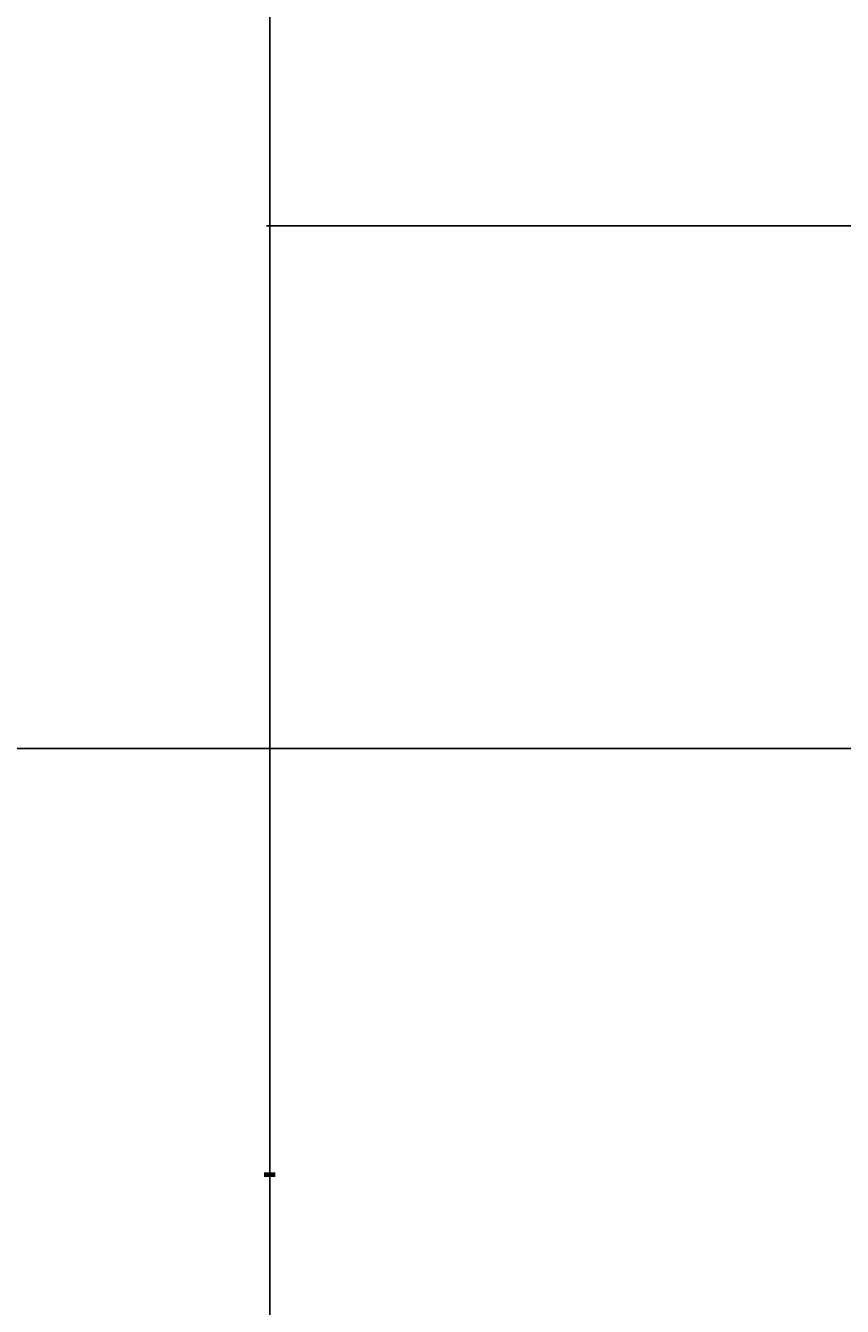
# Model space of a CAD drawing. Units: inches. Extents: x -301 to 715, y -607 to 364.
# Tile 124 of 141: x 148 to 194, y 230 to 303. Entities that reach past the tile are written whole.
import ezdxf

# ---------------------------------------------------------------- set-up
doc = ezdxf.new("R2010")
doc.units = ezdxf.units.IN
doc.header["$MEASUREMENT"] = 0
doc.layers.add('A-ANNO-DIMS', color=2, linetype='Continuous', lineweight=18)
doc.styles.get("Standard").update_dxf_attribs({"font": 'arial.ttf'})
doc.dimstyles.get("Standard").update_dxf_attribs({"dimtxt": 0.18, "dimasz": 0.18, "dimexe": 0.18, "dimexo": 0.0625, "dimgap": 0.09, "dimtad": 0, "dimtih": 1, "dimtoh": 1, "dimdec": 1, "dimzin": 0, "dimdsep": 46, "dimlunit": 4, "dimtxsty": 'Standard', "dimcen": 0.09, "dimclrd": 3, "dimclre": 4, "dimclrt": 6, "dimadec": 0, "dimazin": 0, "dimtfac": 1, "dimtdec": 1, "dimtofl": 0, "dimtmove": 0, "dimatfit": 3, "dimfxl": 1, "dimtfill": 2, "dimtfillclr": 51, "dimtolj": 1, "dimtzin": 0, "dimarcsym": 0})

# ---------------------------------------------------------------- blocks, each defined once
blk = doc.blocks.new('*D153')
at = {"layer": 'A-ANNO-DIMS', "color": 4, "lineweight": -2, "transparency": 16777216}
for p, q in [((132.959, 310.182), (233.659, 310.182)), ((123.959, 193.182), (233.659, 193.182))]:
    blk.add_line(p, q, dxfattribs=at)
at = {"layer": 'A-ANNO-DIMS', "color": 3, "lineweight": -2, "transparency": 16777216}
for p, q in [((233.479, 310.002), (233.479, 251.864)), ((233.479, 193.362), (233.479, 251.5))]:
    blk.add_line(p, q, dxfattribs=at)
at = {"layer": 'A-ANNO-DIMS', "color": 3, "transparency": 16777216}
for points in [[(233.449, 310.002), (233.509, 310.002), (233.479, 310.182)], [(233.449, 193.362), (233.509, 193.362), (233.479, 193.182)]]:
    blk.add_solid(points, dxfattribs=at)
at = {"layer": 'Defpoints', "color": 0, "transparency": 16777216}
for p in [(132.897, 310.182), (123.897, 193.182), (233.479, 193.182)]:
    blk.add_point(p, dxfattribs=at)
at = {"layer": 'A-ANNO-DIMS', "color": 6, "transparency": 16777216, "insert": (233.479, 251.682), "char_height": 0.18, "attachment_point": 5, "bg_fill": 1, "box_fill_scale": 1.25, "bg_fill_color": 51, "bg_fill_transparency": 0}
blk.add_mtext('\\A1;9\'-9"', dxfattribs=at)
blk = doc.blocks.new('*D157')
at = {"layer": 'A-ANNO-DIMS', "color": 4, "lineweight": -2, "transparency": 16777216}
for p, q in [((-50.541, 261.432), (233.659, 261.432)), ((-50.541, 221.682), (233.659, 221.682))]:
    blk.add_line(p, q, dxfattribs=at)
at = {"layer": 'A-ANNO-DIMS', "color": 3, "lineweight": -2, "transparency": 16777216}
for p, q in [((233.479, 261.252), (233.479, 241.739)), ((233.479, 221.862), (233.479, 241.375))]:
    blk.add_line(p, q, dxfattribs=at)
at = {"layer": 'A-ANNO-DIMS', "color": 3, "transparency": 16777216}
for points in [[(233.449, 261.252), (233.509, 261.252), (233.479, 261.432)], [(233.449, 221.862), (233.509, 221.862), (233.479, 221.682)]]:
    blk.add_solid(points, dxfattribs=at)
at = {"layer": 'Defpoints', "color": 0, "transparency": 16777216}
for p in [(-50.603, 261.432), (233.479, 261.432), (-50.603, 221.682)]:
    blk.add_point(p, dxfattribs=at)
at = {"layer": 'A-ANNO-DIMS', "color": 6, "transparency": 16777216, "insert": (233.479, 241.557), "char_height": 0.18, "attachment_point": 5, "bg_fill": 1, "box_fill_scale": 1.25, "bg_fill_color": 51, "bg_fill_transparency": 0}
blk.add_mtext('\\A1;3\'-4"', dxfattribs=at)
blk = doc.blocks.new('*D162')
at = {"layer": 'A-ANNO-DIMS', "color": 4, "lineweight": -2, "transparency": 16777216}
for p, q in [((222.328, 320.182), (161.439, 320.182)), ((222.328, -233.818), (161.439, -233.818))]:
    blk.add_line(p, q, dxfattribs=at)
at = {"layer": 'A-ANNO-DIMS', "color": 3, "lineweight": -2, "transparency": 16777216}
for p, q in [((161.619, 320.002), (161.619, 43.364)), ((161.619, -233.638), (161.619, 43))]:
    blk.add_line(p, q, dxfattribs=at)
at = {"layer": 'A-ANNO-DIMS', "color": 3, "transparency": 16777216}
for points in [[(161.589, 320.002), (161.649, 320.002), (161.619, 320.182)], [(161.589, -233.638), (161.649, -233.638), (161.619, -233.818)]]:
    blk.add_solid(points, dxfattribs=at)
at = {"layer": 'Defpoints', "color": 0, "transparency": 16777216}
for p in [(161.619, 320.182), (222.39, 320.182), (222.39, -233.818)]:
    blk.add_point(p, dxfattribs=at)
at = {"layer": 'A-ANNO-DIMS', "color": 6, "transparency": 16777216, "insert": (161.619, 43.182), "char_height": 0.18, "attachment_point": 5, "bg_fill": 1, "box_fill_scale": 1.25, "bg_fill_color": 51, "bg_fill_transparency": 0}
blk.add_mtext('\\A1;46\'-2"', dxfattribs=at)
blk = doc.blocks.new('*D170')
at = {"layer": 'A-ANNO-DIMS', "color": 4, "lineweight": -2, "transparency": 16777216}
for p, q in [((222.328, 291.182), (161.439, 291.182)), ((222.328, 183.182), (161.439, 183.182))]:
    blk.add_line(p, q, dxfattribs=at)
at = {"layer": 'A-ANNO-DIMS', "color": 3, "lineweight": -2, "transparency": 16777216}
for p, q in [((161.619, 291.002), (161.619, 237.364)), ((161.619, 183.362), (161.619, 237))]:
    blk.add_line(p, q, dxfattribs=at)
at = {"layer": 'A-ANNO-DIMS', "color": 3, "transparency": 16777216}
for points in [[(161.589, 291.002), (161.649, 291.002), (161.619, 291.182)], [(161.589, 183.362), (161.649, 183.362), (161.619, 183.182)]]:
    blk.add_solid(points, dxfattribs=at)
at = {"layer": 'Defpoints', "color": 0, "transparency": 16777216}
for p in [(161.619, 291.182), (222.39, 291.182), (222.39, 183.182)]:
    blk.add_point(p, dxfattribs=at)
at = {"layer": 'A-ANNO-DIMS', "color": 6, "transparency": 16777216, "insert": (161.619, 237.182), "char_height": 0.18, "attachment_point": 5, "bg_fill": 1, "box_fill_scale": 1.25, "bg_fill_color": 51, "bg_fill_transparency": 0}
blk.add_mtext('\\A1;9\'-0"', dxfattribs=at)

msp = doc.modelspace()

# ---------------------------------------------------------------- dimensions: what is measured, and where the dimension line sits
at = {"layer": 'A-ANNO-DIMS'}
for base, p1, p2, picture, middle in [((161.619, 320.182), (222.39, -233.818), (222.39, 320.182), '*D162', (161.619, 43.182)), ((233.479, 193.182), (132.897, 310.182), (123.897, 193.182), '*D153', (233.479, 251.682)), ((161.619, 291.182), (222.39, 183.182), (222.39, 291.182), '*D170', (161.619, 237.182)), ((233.479242, 261.43233), (-50.603288, 221.68233), (-50.603288, 261.43233), '*D157', (233.479242, 241.55733))]:
    dim = msp.add_linear_dim(base=base, p1=p1, p2=p2, angle=90, dimstyle='Standard', override={"dimdec": 1, "dimlfac": 1, "dimrnd": 0, "dimzin": 1, "dimdsep": 46, "dimlunit": 4, "dimfrac": 2}, dxfattribs=at)
    dim.commit()
    dim.dimension.update_dxf_attribs({"geometry": picture, "text_midpoint": middle})

doc.saveas('drawing.dxf')
